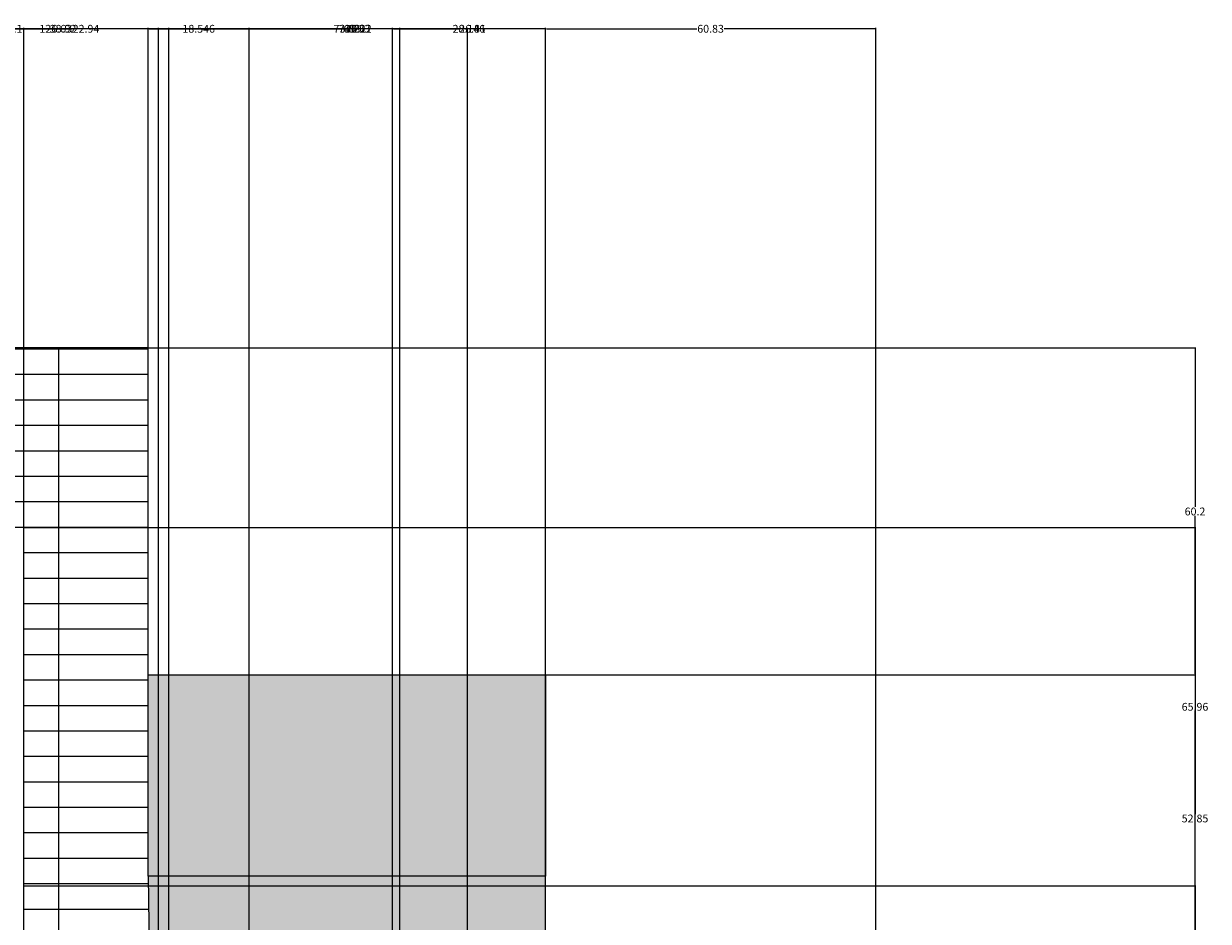
# Model space of a CAD drawing. Units: inches. Extents: x 241 to 943, y 109 to 1396.
# Tile 34 of 34: x 725 to 943, y 1231 to 1396. Entities that reach past the tile are written whole.
import ezdxf

# ---------------------------------------------------------------- set-up
doc = ezdxf.new("R2010")
doc.units = ezdxf.units.IN
doc.header["$MEASUREMENT"] = 0
for name, color, linetype, lineweight in [('A-ANNO-DIMS', 2, 'Continuous', 18), ('A-ELEV', 7, 'Continuous', 25), ('A-ELEV-SHAD', 9, 'Continuous', 13), ('A-WALL-PATT', 8, 'Continuous', 13)]:
    doc.layers.add(name, color=color, linetype=linetype, lineweight=lineweight)
doc.styles.get("Standard").update_dxf_attribs({"font": 'arial.ttf'})
doc.dimstyles.get("Standard").update_dxf_attribs({"dimtxt": 1.4375, "dimasz": 0.18, "dimexe": 0.18, "dimexo": 0.0625, "dimgap": 0.09, "dimtad": 0, "dimtih": 1, "dimtoh": 1, "dimdec": 4, "dimzin": 0, "dimdsep": 46, "dimlunit": 4, "dimtxsty": 'Standard', "dimcen": 0.09, "dimadec": 0, "dimazin": 0, "dimtfac": 1, "dimtdec": 4, "dimtofl": 0, "dimtmove": 0, "dimatfit": 3, "dimfxl": 1, "dimtolj": 1, "dimtzin": 0, "dimarcsym": 0})

# ---------------------------------------------------------------- blocks, each defined once
blk = doc.blocks.new('*D6')
at = {"layer": 'A-ANNO-DIMS', "color": 0, "lineweight": -2, "transparency": 16777216}
for p, q in [((820.84, 232.89), (820.84, 1395.05)), ((821.02, 1394.87), (848.73, 1394.87)), ((881.49, 1394.87), (853.77, 1394.87)), ((881.67, 232.89), (881.67, 1395.05))]:
    blk.add_line(p, q, dxfattribs=at)
at = {"layer": 'A-ANNO-DIMS', "color": 0, "transparency": 16777216}
for points in [[(821.02, 1394.9), (821.02, 1394.84), (820.84, 1394.87)], [(881.49, 1394.9), (881.49, 1394.84), (881.67, 1394.87)]]:
    blk.add_solid(points, dxfattribs=at)
at = {"layer": 'Defpoints', "color": 0, "transparency": 16777216}
for p in [(881.67, 1394.87), (820.84, 232.83), (881.67, 232.83)]:
    blk.add_point(p, dxfattribs=at)
at = {"layer": 'A-ANNO-DIMS', "color": 0, "transparency": 16777216, "insert": (851.25, 1394.87), "char_height": 1.438, "attachment_point": 5}
blk.add_mtext('\\A1;60.83', dxfattribs=at)
blk = doc.blocks.new('*D14')
at = {"layer": 'A-ANNO-DIMS', "color": 0, "lineweight": -2, "transparency": 16777216}
for p, q in [((667.39, 290.06), (667.39, 1395.05)), ((667.57, 1394.87), (727.7, 1394.87)), ((793.85, 1394.87), (733.72, 1394.87)), ((794.03, 290.06), (794.03, 1395.05))]:
    blk.add_line(p, q, dxfattribs=at)
at = {"layer": 'A-ANNO-DIMS', "color": 0, "transparency": 16777216}
for points in [[(667.57, 1394.9), (667.57, 1394.84), (667.39, 1394.87)], [(793.85, 1394.9), (793.85, 1394.84), (794.03, 1394.87)]]:
    blk.add_solid(points, dxfattribs=at)
at = {"layer": 'Defpoints', "color": 0, "transparency": 16777216}
for p in [(794.03, 1394.87), (667.39, 290), (794.03, 290)]:
    blk.add_point(p, dxfattribs=at)
at = {"layer": 'A-ANNO-DIMS', "color": 0, "transparency": 16777216, "insert": (730.71, 1394.87), "char_height": 1.438, "attachment_point": 5}
blk.add_mtext('\\A1;126.63', dxfattribs=at)
blk = doc.blocks.new('*D15')
at = {"layer": 'A-ANNO-DIMS', "color": 0, "lineweight": -2, "transparency": 16777216}
for p, q in [((794.03, 290.06), (794.03, 1395.05)), ((794.21, 1394.87), (805.04, 1394.87)), ((820.66, 1394.87), (809.82, 1394.87)), ((820.84, 232.89), (820.84, 1395.05))]:
    blk.add_line(p, q, dxfattribs=at)
at = {"layer": 'A-ANNO-DIMS', "color": 0, "transparency": 16777216}
for points in [[(794.21, 1394.9), (794.21, 1394.84), (794.03, 1394.87)], [(820.66, 1394.9), (820.66, 1394.84), (820.84, 1394.87)]]:
    blk.add_solid(points, dxfattribs=at)
at = {"layer": 'Defpoints', "color": 0, "transparency": 16777216}
for p in [(820.84, 1394.87), (794.03, 290), (820.84, 232.83)]:
    blk.add_point(p, dxfattribs=at)
at = {"layer": 'A-ANNO-DIMS', "color": 0, "transparency": 16777216, "insert": (807.43, 1394.87), "char_height": 1.438, "attachment_point": 5}
blk.add_mtext('\\A1;26.81', dxfattribs=at)
blk = doc.blocks.new('*D18')
at = {"layer": 'A-ANNO-DIMS', "color": 0, "lineweight": -2, "transparency": 16777216}
for p, q in [((508.31, 1336.18), (508.31, 1395.05)), ((508.49, 1394.87), (624.94, 1394.87)), ((747.58, 1394.87), (631.12, 1394.87)), ((747.76, 1336.18), (747.76, 1395.05))]:
    blk.add_line(p, q, dxfattribs=at)
at = {"layer": 'A-ANNO-DIMS', "color": 0, "transparency": 16777216}
for points in [[(508.49, 1394.9), (508.49, 1394.84), (508.31, 1394.87)], [(747.58, 1394.9), (747.58, 1394.84), (747.76, 1394.87)]]:
    blk.add_solid(points, dxfattribs=at)
at = {"layer": 'Defpoints', "color": 0, "transparency": 16777216}
for p in [(747.76, 1394.87), (508.31, 1336.12), (747.76, 1336.12)]:
    blk.add_point(p, dxfattribs=at)
at = {"layer": 'A-ANNO-DIMS', "color": 0, "transparency": 16777216, "insert": (628.03, 1394.87), "char_height": 1.438, "attachment_point": 5}
blk.add_mtext('\\A1;239.45', dxfattribs=at)
blk = doc.blocks.new('*D19')
at = {"layer": 'A-ANNO-DIMS', "color": 0, "lineweight": -2, "transparency": 16777216}
for p, q in [((747.76, 1275.98), (747.76, 1395.05)), ((747.94, 1394.87), (781.79, 1394.87)), ((820.66, 1394.87), (786.81, 1394.87)), ((820.84, 1275.98), (820.84, 1395.05))]:
    blk.add_line(p, q, dxfattribs=at)
at = {"layer": 'A-ANNO-DIMS', "color": 0, "transparency": 16777216}
for points in [[(747.94, 1394.9), (747.94, 1394.84), (747.76, 1394.87)], [(820.66, 1394.9), (820.66, 1394.84), (820.84, 1394.87)]]:
    blk.add_solid(points, dxfattribs=at)
at = {"layer": 'Defpoints', "color": 0, "transparency": 16777216}
for p in [(820.84, 1394.87), (747.76, 1275.91), (820.84, 1275.91)]:
    blk.add_point(p, dxfattribs=at)
at = {"layer": 'A-ANNO-DIMS', "color": 0, "transparency": 16777216, "insert": (784.3, 1394.87), "char_height": 1.438, "attachment_point": 5}
blk.add_mtext('\\A1;73.08', dxfattribs=at)
blk = doc.blocks.new('*D42')
at = {"layer": 'A-ANNO-DIMS', "color": 0, "lineweight": -2, "transparency": 16777216}
for p, q in [((820.9, 1275.91), (940.6, 1275.91)), ((940.42, 1275.73), (940.42, 1250.31)), ((940.42, 1223.24), (940.42, 1248.66)), ((820.9, 1223.06), (940.6, 1223.06))]:
    blk.add_line(p, q, dxfattribs=at)
at = {"layer": 'A-ANNO-DIMS', "color": 0, "transparency": 16777216}
for points in [[(940.39, 1275.73), (940.45, 1275.73), (940.42, 1275.91)], [(940.39, 1223.24), (940.45, 1223.24), (940.42, 1223.06)]]:
    blk.add_solid(points, dxfattribs=at)
at = {"layer": 'Defpoints', "color": 0, "transparency": 16777216}
for p in [(820.84, 1275.91), (940.42, 1275.91), (820.84, 1223.06)]:
    blk.add_point(p, dxfattribs=at)
at = {"layer": 'A-ANNO-DIMS', "color": 0, "transparency": 16777216, "insert": (940.42, 1249.49), "char_height": 1.438, "attachment_point": 5}
blk.add_mtext('\\A1;52.85', dxfattribs=at)
blk = doc.blocks.new('*D43')
at = {"layer": 'A-ANNO-DIMS', "color": 0, "lineweight": -2, "transparency": 16777216}
for p, q in [((747.82, 1336.12), (940.6, 1336.12)), ((940.42, 1335.94), (940.42, 1306.84)), ((940.42, 1276.09), (940.42, 1305.19)), ((747.82, 1275.91), (940.6, 1275.91))]:
    blk.add_line(p, q, dxfattribs=at)
at = {"layer": 'A-ANNO-DIMS', "color": 0, "transparency": 16777216}
for points in [[(940.39, 1335.94), (940.45, 1335.94), (940.42, 1336.12)], [(940.39, 1276.09), (940.45, 1276.09), (940.42, 1275.91)]]:
    blk.add_solid(points, dxfattribs=at)
at = {"layer": 'Defpoints', "color": 0, "transparency": 16777216}
for p in [(747.76, 1336.12), (940.42, 1336.12), (747.76, 1275.91)]:
    blk.add_point(p, dxfattribs=at)
at = {"layer": 'A-ANNO-DIMS', "color": 0, "transparency": 16777216, "insert": (940.42, 1306.01), "char_height": 1.438, "attachment_point": 5}
blk.add_mtext('\\A1;60.2', dxfattribs=at)
blk = doc.blocks.new('*D54')
at = {"layer": 'A-ANNO-DIMS', "color": 0, "lineweight": -2, "transparency": 16777216}
for p, q in [((724.88, 1237.07), (940.6, 1237.07)), ((940.42, 1236.89), (940.42, 1208.23)), ((940.42, 1177.91), (940.42, 1206.58)), ((724.88, 1177.73), (940.6, 1177.73))]:
    blk.add_line(p, q, dxfattribs=at)
at = {"layer": 'A-ANNO-DIMS', "color": 0, "transparency": 16777216}
for points in [[(940.39, 1236.89), (940.45, 1236.89), (940.42, 1237.07)], [(940.39, 1177.91), (940.45, 1177.91), (940.42, 1177.73)]]:
    blk.add_solid(points, dxfattribs=at)
at = {"layer": 'Defpoints', "color": 0, "transparency": 16777216}
for p in [(724.82, 1237.07), (940.42, 1237.07), (724.82, 1177.73)]:
    blk.add_point(p, dxfattribs=at)
at = {"layer": 'A-ANNO-DIMS', "color": 0, "transparency": 16777216, "insert": (940.42, 1207.4), "char_height": 1.438, "attachment_point": 5}
blk.add_mtext('\\A1;59.34', dxfattribs=at)
blk = doc.blocks.new('*D55')
at = {"layer": 'A-ANNO-DIMS', "color": 0, "lineweight": -2, "transparency": 16777216}
for p, q in [((724.88, 1303.03), (940.6, 1303.03)), ((940.42, 1302.85), (940.42, 1270.87)), ((940.42, 1237.25), (940.42, 1269.23)), ((724.88, 1237.07), (940.6, 1237.07))]:
    blk.add_line(p, q, dxfattribs=at)
at = {"layer": 'A-ANNO-DIMS', "color": 0, "transparency": 16777216}
for points in [[(940.39, 1302.85), (940.45, 1302.85), (940.42, 1303.03)], [(940.39, 1237.25), (940.45, 1237.25), (940.42, 1237.07)]]:
    blk.add_solid(points, dxfattribs=at)
at = {"layer": 'Defpoints', "color": 0, "transparency": 16777216}
for p in [(724.82, 1303.03), (940.42, 1303.03), (724.82, 1237.07)]:
    blk.add_point(p, dxfattribs=at)
at = {"layer": 'A-ANNO-DIMS', "color": 0, "transparency": 16777216, "insert": (940.42, 1270.05), "char_height": 1.438, "attachment_point": 5}
blk.add_mtext('\\A1;65.96', dxfattribs=at)
blk = doc.blocks.new('*D56')
at = {"layer": 'A-ANNO-DIMS', "color": 0, "lineweight": -2, "transparency": 16777216}
for p, q in [((533.95, 1303.09), (533.95, 1395.05)), ((534.13, 1394.87), (626.38, 1394.87)), ((724.64, 1394.87), (632.39, 1394.87)), ((724.82, 1303.09), (724.82, 1395.05))]:
    blk.add_line(p, q, dxfattribs=at)
at = {"layer": 'A-ANNO-DIMS', "color": 0, "transparency": 16777216}
for points in [[(534.13, 1394.9), (534.13, 1394.84), (533.95, 1394.87)], [(724.64, 1394.9), (724.64, 1394.84), (724.82, 1394.87)]]:
    blk.add_solid(points, dxfattribs=at)
at = {"layer": 'Defpoints', "color": 0, "transparency": 16777216}
for p in [(724.82, 1394.87), (533.95, 1303.03), (724.82, 1303.03)]:
    blk.add_point(p, dxfattribs=at)
at = {"layer": 'A-ANNO-DIMS', "color": 0, "transparency": 16777216, "insert": (629.39, 1394.87), "char_height": 1.438, "attachment_point": 5}
blk.add_mtext('\\A1;190.87', dxfattribs=at)
blk = doc.blocks.new('*D58')
at = {"layer": 'A-ANNO-DIMS', "color": 0, "lineweight": -2, "transparency": 16777216}
for p, q in [((766.3, 1177.6), (766.3, 1395.05)), ((766.48, 1394.87), (783.88, 1394.87)), ((806.35, 1394.87), (788.95, 1394.87)), ((806.53, 1177.6), (806.53, 1395.05))]:
    blk.add_line(p, q, dxfattribs=at)
at = {"layer": 'A-ANNO-DIMS', "color": 0, "transparency": 16777216}
for points in [[(766.48, 1394.9), (766.48, 1394.84), (766.3, 1394.87)], [(806.35, 1394.9), (806.35, 1394.84), (806.53, 1394.87)]]:
    blk.add_solid(points, dxfattribs=at)
at = {"layer": 'Defpoints', "color": 0, "transparency": 16777216}
for p in [(806.53, 1394.87), (766.3, 1177.54), (806.53, 1177.54)]:
    blk.add_point(p, dxfattribs=at)
at = {"layer": 'A-ANNO-DIMS', "color": 0, "transparency": 16777216, "insert": (786.42, 1394.87), "char_height": 1.438, "attachment_point": 5}
blk.add_mtext('\\A1;40.22', dxfattribs=at)
blk = doc.blocks.new('*D63')
at = {"layer": 'A-ANNO-DIMS', "color": 0, "lineweight": -2, "transparency": 16777216}
for p, q in [((651.6, 568.89), (651.6, 1395.05)), ((651.78, 1394.87), (719.84, 1394.87)), ((792.51, 1394.87), (724.45, 1394.87)), ((792.69, 568.89), (792.69, 1395.05))]:
    blk.add_line(p, q, dxfattribs=at)
at = {"layer": 'A-ANNO-DIMS', "color": 0, "transparency": 16777216}
for points in [[(651.78, 1394.9), (651.78, 1394.84), (651.6, 1394.87)], [(792.51, 1394.9), (792.51, 1394.84), (792.69, 1394.87)]]:
    blk.add_solid(points, dxfattribs=at)
at = {"layer": 'Defpoints', "color": 0, "transparency": 16777216}
for p in [(792.69, 1394.87), (651.6, 568.83), (792.69, 568.83)]:
    blk.add_point(p, dxfattribs=at)
at = {"layer": 'A-ANNO-DIMS', "color": 0, "transparency": 16777216, "insert": (722.14, 1394.87), "char_height": 1.438, "attachment_point": 5}
blk.add_mtext('\\A1;141.1', dxfattribs=at)
blk = doc.blocks.new('*D64')
at = {"layer": 'A-ANNO-DIMS', "color": 0, "lineweight": -2, "transparency": 16777216}
for p, q in [((792.69, 568.89), (792.69, 1395.05)), ((792.87, 1394.87), (803.68, 1394.87)), ((820.66, 1394.87), (809.85, 1394.87)), ((820.84, 568.89), (820.84, 1395.05))]:
    blk.add_line(p, q, dxfattribs=at)
at = {"layer": 'A-ANNO-DIMS', "color": 0, "transparency": 16777216}
for points in [[(792.87, 1394.9), (792.87, 1394.84), (792.69, 1394.87)], [(820.66, 1394.9), (820.66, 1394.84), (820.84, 1394.87)]]:
    blk.add_solid(points, dxfattribs=at)
at = {"layer": 'Defpoints', "color": 0, "transparency": 16777216}
for p in [(820.84, 1394.87), (792.69, 568.83), (820.84, 568.83)]:
    blk.add_point(p, dxfattribs=at)
at = {"layer": 'A-ANNO-DIMS', "color": 0, "transparency": 16777216, "insert": (806.76, 1394.87), "char_height": 1.438, "attachment_point": 5}
blk.add_mtext('\\A1;28.146', dxfattribs=at)
blk = doc.blocks.new('*D66')
at = {"layer": 'A-ANNO-DIMS', "color": 0, "lineweight": -2, "transparency": 16777216}
for p, q in [((617.76, 702.85), (617.76, 1395.05)), ((617.94, 1394.87), (680.69, 1394.87)), ((749.45, 1394.87), (686.7, 1394.87)), ((749.63, 702.85), (749.63, 1395.05))]:
    blk.add_line(p, q, dxfattribs=at)
at = {"layer": 'A-ANNO-DIMS', "color": 0, "transparency": 16777216}
for points in [[(617.94, 1394.9), (617.94, 1394.84), (617.76, 1394.87)], [(749.45, 1394.9), (749.45, 1394.84), (749.63, 1394.87)]]:
    blk.add_solid(points, dxfattribs=at)
at = {"layer": 'Defpoints', "color": 0, "transparency": 16777216}
for p in [(749.63, 1394.87), (617.76, 702.79), (749.63, 702.79)]:
    blk.add_point(p, dxfattribs=at)
at = {"layer": 'A-ANNO-DIMS', "color": 0, "transparency": 16777216, "insert": (683.7, 1394.87), "char_height": 1.438, "attachment_point": 5}
blk.add_mtext('\\A1;131.87', dxfattribs=at)
blk = doc.blocks.new('*D68')
at = {"layer": 'A-ANNO-DIMS', "color": 0, "lineweight": -2, "transparency": 16777216}
for p, q in [((617.76, 841.6), (617.76, 1395.05)), ((617.94, 1394.87), (702.22, 1394.87)), ((792.51, 1394.87), (708.23, 1394.87)), ((792.69, 841.6), (792.69, 1395.05))]:
    blk.add_line(p, q, dxfattribs=at)
at = {"layer": 'A-ANNO-DIMS', "color": 0, "transparency": 16777216}
for points in [[(617.94, 1394.9), (617.94, 1394.84), (617.76, 1394.87)], [(792.51, 1394.9), (792.51, 1394.84), (792.69, 1394.87)]]:
    blk.add_solid(points, dxfattribs=at)
at = {"layer": 'Defpoints', "color": 0, "transparency": 16777216}
for p in [(792.69, 1394.87), (617.76, 841.54), (792.69, 841.54)]:
    blk.add_point(p, dxfattribs=at)
at = {"layer": 'A-ANNO-DIMS', "color": 0, "transparency": 16777216, "insert": (705.23, 1394.87), "char_height": 1.438, "attachment_point": 5}
blk.add_mtext('\\A1;174.93', dxfattribs=at)
blk = doc.blocks.new('*D70')
at = {"layer": 'A-ANNO-DIMS', "color": 0, "lineweight": -2, "transparency": 16777216}
for p, q in [((603.87, 1009.6), (603.87, 1395.05)), ((604.05, 1394.87), (674.69, 1394.87)), ((751.33, 1394.87), (680.69, 1394.87)), ((751.51, 1009.6), (751.51, 1395.05))]:
    blk.add_line(p, q, dxfattribs=at)
at = {"layer": 'A-ANNO-DIMS', "color": 0, "transparency": 16777216}
for points in [[(604.05, 1394.9), (604.05, 1394.84), (603.87, 1394.87)], [(751.33, 1394.9), (751.33, 1394.84), (751.51, 1394.87)]]:
    blk.add_solid(points, dxfattribs=at)
at = {"layer": 'Defpoints', "color": 0, "transparency": 16777216}
for p in [(751.51, 1394.87), (603.87, 1009.54), (751.51, 1009.54)]:
    blk.add_point(p, dxfattribs=at)
at = {"layer": 'A-ANNO-DIMS', "color": 0, "transparency": 16777216, "insert": (677.69, 1394.87), "char_height": 1.438, "attachment_point": 5}
blk.add_mtext('\\A1;147.64', dxfattribs=at)
blk = doc.blocks.new('*D71')
at = {"layer": 'A-ANNO-DIMS', "color": 0, "lineweight": -2, "transparency": 16777216}
for p, q in [((751.51, 902.92), (751.51, 1395.05)), ((751.69, 1394.87), (783.65, 1394.87)), ((820.66, 1394.87), (788.69, 1394.87)), ((820.84, 902.92), (820.84, 1395.05))]:
    blk.add_line(p, q, dxfattribs=at)
at = {"layer": 'A-ANNO-DIMS', "color": 0, "transparency": 16777216}
for points in [[(751.69, 1394.9), (751.69, 1394.84), (751.51, 1394.87)], [(820.66, 1394.9), (820.66, 1394.84), (820.84, 1394.87)]]:
    blk.add_solid(points, dxfattribs=at)
at = {"layer": 'Defpoints', "color": 0, "transparency": 16777216}
for p in [(820.84, 1394.87), (751.51, 902.85), (820.84, 902.85)]:
    blk.add_point(p, dxfattribs=at)
at = {"layer": 'A-ANNO-DIMS', "color": 0, "transparency": 16777216, "insert": (786.17, 1394.87), "char_height": 1.438, "attachment_point": 5}
blk.add_mtext('\\A1;69.33', dxfattribs=at)
blk = doc.blocks.new('*D84')
at = {"layer": 'A-ANNO-DIMS', "color": 0, "lineweight": -2, "transparency": 16777216}
for p, q in [((749.63, 702.85), (749.63, 1395.05)), ((749.81, 1394.87), (782.73, 1394.87)), ((820.66, 1394.87), (787.74, 1394.87)), ((820.84, 736.89), (820.84, 1395.05))]:
    blk.add_line(p, q, dxfattribs=at)
at = {"layer": 'A-ANNO-DIMS', "color": 0, "transparency": 16777216}
for points in [[(749.81, 1394.9), (749.81, 1394.84), (749.63, 1394.87)], [(820.66, 1394.9), (820.66, 1394.84), (820.84, 1394.87)]]:
    blk.add_solid(points, dxfattribs=at)
at = {"layer": 'Defpoints', "color": 0, "transparency": 16777216}
for p in [(820.84, 1394.87), (820.84, 736.83), (749.63, 702.79)]:
    blk.add_point(p, dxfattribs=at)
at = {"layer": 'A-ANNO-DIMS', "color": 0, "transparency": 16777216, "insert": (785.24, 1394.87), "char_height": 1.438, "attachment_point": 5}
blk.add_mtext('\\A1;71.20', dxfattribs=at)
blk = doc.blocks.new('*D93')
at = {"layer": 'A-ANNO-DIMS', "color": 0, "lineweight": -2, "transparency": 16777216}
for p, q in [((724.82, 1303.09), (724.82, 1395.05)), ((725, 1394.87), (733.76, 1394.87)), ((747.58, 1394.87), (738.81, 1394.87)), ((747.76, 1275.98), (747.76, 1395.05))]:
    blk.add_line(p, q, dxfattribs=at)
at = {"layer": 'A-ANNO-DIMS', "color": 0, "transparency": 16777216}
for points in [[(725, 1394.9), (725, 1394.84), (724.82, 1394.87)], [(747.58, 1394.9), (747.58, 1394.84), (747.76, 1394.87)]]:
    blk.add_solid(points, dxfattribs=at)
at = {"layer": 'Defpoints', "color": 0, "transparency": 16777216}
for p in [(747.76, 1394.87), (724.82, 1303.03), (747.76, 1275.91)]:
    blk.add_point(p, dxfattribs=at)
at = {"layer": 'A-ANNO-DIMS', "color": 0, "transparency": 16777216, "insert": (736.29, 1394.87), "char_height": 1.438, "attachment_point": 5}
blk.add_mtext('\\A1;22.94', dxfattribs=at)
blk = doc.blocks.new('*D94')
at = {"layer": 'A-ANNO-DIMS', "color": 0, "lineweight": -2, "transparency": 16777216}
for p, q in [((747.76, 1275.98), (747.76, 1395.05)), ((747.94, 1394.87), (754.03, 1394.87)), ((766.12, 1394.87), (760.04, 1394.87)), ((766.3, 1103.11), (766.3, 1395.05))]:
    blk.add_line(p, q, dxfattribs=at)
at = {"layer": 'A-ANNO-DIMS', "color": 0, "transparency": 16777216}
for points in [[(747.94, 1394.9), (747.94, 1394.84), (747.76, 1394.87)], [(766.12, 1394.9), (766.12, 1394.84), (766.3, 1394.87)]]:
    blk.add_solid(points, dxfattribs=at)
at = {"layer": 'Defpoints', "color": 0, "transparency": 16777216}
for p in [(766.3, 1394.87), (747.76, 1275.91), (766.3, 1103.05)]:
    blk.add_point(p, dxfattribs=at)
at = {"layer": 'A-ANNO-DIMS', "color": 0, "transparency": 16777216, "insert": (757.03, 1394.87), "char_height": 1.438, "attachment_point": 5}
blk.add_mtext('\\A1;18.546', dxfattribs=at)
blk = doc.blocks.new('*D109')
at = {"layer": 'A-ANNO-DIMS', "color": 0, "lineweight": -2, "transparency": 16777216}
for p, q in [((682.87, 1110.23), (682.87, 1395.05)), ((683.05, 1394.87), (701.31, 1394.87)), ((724.64, 1394.87), (706.39, 1394.87)), ((724.82, 1108.23), (724.82, 1395.05))]:
    blk.add_line(p, q, dxfattribs=at)
at = {"layer": 'A-ANNO-DIMS', "color": 0, "transparency": 16777216}
for points in [[(683.05, 1394.9), (683.05, 1394.84), (682.87, 1394.87)], [(724.64, 1394.9), (724.64, 1394.84), (724.82, 1394.87)]]:
    blk.add_solid(points, dxfattribs=at)
at = {"layer": 'Defpoints', "color": 0, "transparency": 16777216}
for p in [(724.82, 1394.87), (682.87, 1110.17), (724.82, 1108.17)]:
    blk.add_point(p, dxfattribs=at)
at = {"layer": 'A-ANNO-DIMS', "color": 0, "transparency": 16777216, "insert": (703.85, 1394.87), "char_height": 1.438, "attachment_point": 5}
blk.add_mtext('\\A1;41.94', dxfattribs=at)
blk = doc.blocks.new('*D117')
at = {"layer": 'A-ANNO-DIMS', "color": 0, "lineweight": -2, "transparency": 16777216}
for p, q in [((712.58, 902.92), (712.58, 1395.05)), ((712.76, 1394.87), (729.54, 1394.87)), ((751.33, 1394.87), (734.55, 1394.87)), ((751.51, 902.92), (751.51, 1395.05))]:
    blk.add_line(p, q, dxfattribs=at)
at = {"layer": 'A-ANNO-DIMS', "color": 0, "transparency": 16777216}
for points in [[(712.76, 1394.9), (712.76, 1394.84), (712.58, 1394.87)], [(751.33, 1394.9), (751.33, 1394.84), (751.51, 1394.87)]]:
    blk.add_solid(points, dxfattribs=at)
at = {"layer": 'Defpoints', "color": 0, "transparency": 16777216}
for p in [(751.51, 1394.87), (712.58, 902.85), (751.51, 902.85)]:
    blk.add_point(p, dxfattribs=at)
at = {"layer": 'A-ANNO-DIMS', "color": 0, "transparency": 16777216, "insert": (732.05, 1394.87), "char_height": 1.438, "attachment_point": 5}
blk.add_mtext('\\A1;38.92', dxfattribs=at)

msp = doc.modelspace()

# ---------------------------------------------------------------- hatches: boundary and pattern name
at = {"layer": 'A-ELEV-SHAD'}
h = msp.add_hatch(color=256, dxfattribs=at)
h.dxf.hatch_style = 1
h.paths.add_polyline_path([(508.3064, 1070.8538), (377.0391, 1070.8538), (377.0391, 1009.5382), (508.3064, 1009.5382)])
h.paths.add_polyline_path([(508.3064, 1238.8538), (377.0391, 1238.8538), (377.0391, 1177.5382), (508.3064, 1177.5382)])
h.paths.add_polyline_path([(581.3632, 902.8538), (568.1348, 902.8538), (553.5166, 902.8538), (377.0391, 902.8538), (377.0391, 841.5382), (553.5166, 841.5382), (564.8076, 841.5382), (581.3632, 841.5382)])
h.paths.add_polyline_path([(820.8374, 1275.9142), (747.7579, 1275.9142), (747.7579, 1238.8538), (820.8374, 1238.8538)])
h.paths.add_polyline_path([(820.8374, 1238.8538), (747.7579, 1238.8538), (747.9341, 1223.0633), (820.8374, 1223.0633)])
h.paths.add_polyline_path([(396.3125, 841.5382), (377.0391, 841.5382), (377.0391, 734.8538), (389.0429, 734.8538), (389.0429, 735.188), (389.0429, 773.4916), (396.3125, 773.4916), (396.3125, 780.5808), (390.5597, 780.5808), (388.0428, 780.5808, -1), (388.0428, 782.5808), (390.5597, 782.5808), (396.3125, 782.5808)])
at = {"layer": 'A-WALL-PATT'}
h = msp.add_hatch(dxfattribs=at)
h.set_pattern_fill('GRATE', color=256, scale=150)
h.paths.add_polyline_path([(747.7579, 1238.8538), (747.7579, 1275.9142), (747.7579, 1336.1154), (508.3064, 1336.1154), (508.3064, 1275.9142), (508.3064, 1238.8538), (508.3064, 1177.5382), (508.3064, 1109.4916), (508.3064, 1070.8538), (553.5166, 1070.8538), (749.6328, 1070.8538)])
h.paths.add_polyline_path([(533.952, 1108.1686), (533.952, 1177.7336), (533.952, 1303.0286), (724.819, 1303.0286), (724.819, 1108.1686)], flags=16)
h.paths.add_polyline_path([(535.952, 1110.1686), (535.952, 1175.7336), (722.819, 1175.7336), (722.819, 1110.1686)], flags=0)
h.paths.add_polyline_path([(643.4534, 1134.0739), (622.521, 1134.0739), (622.521, 1136.0739), (643.4534, 1136.0739)], flags=0)
h.paths.add_polyline_path([(617.7594, 568.8295), (617.7594, 734.8538), (377.0391, 734.8538), (377.0391, 566.8538), (377.0391, 400.8295), (417.0913, 400.8295), (618.9643, 400.8295)])
h.paths.add_polyline_path([(424.1086, 496.4395), (424.1086, 568.8295), (565.2023, 568.8295), (565.2023, 496.4395)], flags=16)
h.paths.add_polyline_path([(426.1086, 498.4395), (426.1086, 566.8295), (563.2023, 566.8295), (563.2023, 508.9074), (563.2023, 498.4395)], flags=0)
h.paths.add_polyline_path([(508.0803, 508.9074), (508.0803, 519.3754), (450.9259, 519.3754), (450.9259, 525.3816), (445.5808, 525.3816, -1), (445.5808, 527.3816), (450.9259, 527.3816), (450.9259, 566.8295), (508.0803, 566.8295), (537.4269, 566.8295), (537.4269, 508.9074)], flags=0)
h.paths.add_polyline_path([(506.0803, 521.3754), (452.9259, 521.3754), (452.9259, 564.8295), (506.0803, 564.8295)], flags=0)
h.paths.add_polyline_path([(424.1086, 628.4013), (424.1086, 700.7912), (592.9542, 700.7912), (592.9542, 628.4013)], flags=16)
h.paths.add_polyline_path([(426.1086, 630.4013), (426.1086, 698.7912), (590.8792, 698.7912), (590.8792, 630.4013)], flags=0)
h.paths.add_polyline_path([(508.1906, 651.3371), (508.0803, 651.3371), (450.9259, 651.3371), (428.0291, 651.3371), (428.0291, 698.7912), (451.9767, 698.7912), (508.0803, 698.7912), (537.4269, 698.7912), (563.2023, 698.7912), (563.2023, 659.3434), (563.9297, 659.3434), (563.9297, 651.3371)], flags=0)
h.paths.add_polyline_path([(506.0803, 653.3371), (452.9259, 653.3371), (452.9259, 657.3434), (445.5808, 657.3434, -1), (445.5808, 659.3434), (452.9259, 659.3434), (452.9259, 696.7912), (506.0803, 696.7912)], flags=0)

# ---------------------------------------------------------------- linework, layer by layer
at = {"layer": 'A-ELEV'}
for p, q in [((747.7579, 1336.1154), (508.3064, 1336.1154)), ((747.7579, 1275.9142), (747.7579, 1336.1154)), ((747.7579, 1238.8538), (747.7579, 1275.9142)), ((747.7579, 1275.9142), (820.8374, 1275.9142)), ((820.8374, 1275.9142), (820.8374, 1238.8538)), ((820.8374, 1238.8538), (747.7579, 1238.8538)), ((747.7579, 1238.8538), (749.6328, 1070.8538)), ((820.8374, 1070.8538), (820.8374, 1238.8538))]:
    msp.add_line(p, q, dxfattribs=at)

# ---------------------------------------------------------------- dimensions: what is measured, and where the dimension line sits
at = {"layer": 'A-ANNO-DIMS'}
for base, p1, p2, override, picture, middle in [((747.7579, 1394.8654), (508.3064, 1336.1154), (747.7579, 1336.1154), {"dimdec": 2, "dimlfac": 1, "dimrnd": 0, "dimzin": 0, "dimdsep": 46, "dimlunit": 2}, '*D18', (628.0322, 1394.8654)), ((724.819, 1394.8654), (533.952, 1303.0286), (724.819, 1303.0286), {"dimdec": 2, "dimlfac": 1, "dimrnd": 0, "dimzin": 0, "dimdsep": 46, "dimlunit": 2}, '*D56', (629.3855, 1394.8654)), ((751.5078, 1394.8654), (603.8694, 1009.5382), (751.5078, 1009.5382), {"dimdec": 2, "dimlfac": 1, "dimrnd": 0, "dimzin": 0, "dimdsep": 46, "dimlunit": 2}, '*D70', (677.6886, 1394.8654)), ((749.6328, 1394.8654), (617.7594, 702.7912), (749.6328, 702.7912), {"dimdec": 2, "dimlfac": 1, "dimrnd": 0, "dimzin": 0, "dimdsep": 46, "dimlunit": 2}, '*D66', (683.6961, 1394.8654)), ((792.691, 1394.8654), (617.7594, 841.5382), (792.691, 841.5382), {"dimdec": 2, "dimlfac": 1, "dimrnd": 0, "dimzin": 0, "dimdsep": 46, "dimlunit": 2}, '*D68', (705.2252, 1394.8654)), ((792.691, 1394.8654), (651.5974, 568.8295), (792.691, 568.8295), {"dimdec": 1, "dimlfac": 1, "dimrnd": 0, "dimzin": 0, "dimdsep": 46, "dimlunit": 2}, '*D63', (722.1442, 1394.8654)), ((794.0275, 1394.8654), (667.3935, 289.9984), (794.0275, 289.9984), {"dimdec": 2, "dimlfac": 1, "dimrnd": 0, "dimzin": 0, "dimdsep": 46, "dimlunit": 2}, '*D14', (730.7105, 1394.8654)), ((724.819, 1394.8654), (682.8748, 1110.1686), (724.819, 1108.1686), {"dimdec": 2, "dimlfac": 1, "dimrnd": 0, "dimzin": 0, "dimdsep": 46, "dimlunit": 2}, '*D109', (703.8469, 1394.8654)), ((751.5078, 1394.8654), (712.5839, 902.8538), (751.5078, 902.8538), {"dimdec": 2, "dimlfac": 1, "dimrnd": 0, "dimzin": 0, "dimdsep": 46, "dimlunit": 2}, '*D117', (732.0459, 1394.8654)), ((747.7579, 1394.8654), (724.819, 1303.0286), (747.7579, 1275.9142), {"dimdec": 2, "dimlfac": 1, "dimrnd": 0, "dimzin": 0, "dimdsep": 46, "dimlunit": 2}, '*D93', (736.2885, 1394.8654)), ((820.8374, 1394.8654), (747.7579, 1275.9142), (820.8374, 1275.9142), {"dimdec": 2, "dimlfac": 1, "dimrnd": 0, "dimzin": 0, "dimdsep": 46, "dimlunit": 2}, '*D19', (784.2976, 1394.8654)), ((766.3038, 1394.8654), (747.7579, 1275.9142), (766.3038, 1103.0477), {"dimdec": 3, "dimlfac": 1, "dimrnd": 0, "dimzin": 0, "dimdsep": 46, "dimlunit": 2}, '*D94', (757.0309, 1394.8654)), ((820.8374, 1394.8654), (749.6328, 702.7912), (820.8374, 736.8295), {"dimdec": 2, "dimlfac": 1, "dimrnd": 0, "dimzin": 0, "dimdsep": 46, "dimlunit": 2}, '*D84', (785.2351, 1394.8654)), ((820.8374, 1394.8654), (751.5078, 902.8538), (820.8374, 902.8538), {"dimdec": 2, "dimlfac": 1, "dimrnd": 0, "dimzin": 0, "dimdsep": 46, "dimlunit": 2}, '*D71', (786.1726, 1394.8654)), ((806.5268, 1394.8654), (766.3038, 1177.5382), (806.5268, 1177.5382), {"dimdec": 2, "dimlfac": 1, "dimrnd": 0, "dimzin": 0, "dimdsep": 46, "dimlunit": 2}, '*D58', (786.4153, 1394.8654)), ((820.8374, 1394.8654), (792.691, 568.8295), (820.8374, 568.8295), {"dimdec": 3, "dimlfac": 1, "dimrnd": 0, "dimzin": 0, "dimdsep": 46, "dimlunit": 2}, '*D64', (806.7642, 1394.8654)), ((820.8374, 1394.8654), (794.0275, 289.9984), (820.8374, 232.8295), {"dimdec": 2, "dimlfac": 1, "dimrnd": 0, "dimzin": 0, "dimdsep": 46, "dimlunit": 2}, '*D15', (807.4324, 1394.8654)), ((881.667, 1394.8654), (820.8374, 232.8295), (881.667, 232.8295), {"dimdec": 2, "dimlfac": 1, "dimrnd": 0, "dimzin": 0, "dimdsep": 46, "dimlunit": 2}, '*D6', (851.2522, 1394.8654))]:
    dim = msp.add_linear_dim(base=base, p1=p1, p2=p2, dimstyle='Standard', override=override, dxfattribs=at)
    dim.commit()
    dim.dimension.update_dxf_attribs({"geometry": picture, "text_midpoint": middle})
for base, p1, p2, override, picture, middle in [((940.417, 1336.1154), (747.7579, 1275.9142), (747.7579, 1336.1154), {"dimdec": 1, "dimlfac": 1, "dimrnd": 0, "dimzin": 0, "dimdsep": 46, "dimlunit": 2}, '*D43', (940.417, 1306.0148)), ((940.417, 1303.0286), (724.819, 1237.0695), (724.819, 1303.0286), {"dimdec": 2, "dimlfac": 1, "dimrnd": 0, "dimzin": 0, "dimdsep": 46, "dimlunit": 2}, '*D55', (940.417, 1270.049)), ((940.417, 1275.9142), (820.8374, 1223.0633), (820.8374, 1275.9142), {"dimdec": 2, "dimlfac": 1, "dimrnd": 0, "dimzin": 0, "dimdsep": 46, "dimlunit": 2}, '*D42', (940.417, 1249.4888)), ((940.417, 1237.0695), (724.819, 1177.7336), (724.819, 1237.0695), {"dimdec": 2, "dimlfac": 1, "dimrnd": 0, "dimzin": 0, "dimdsep": 46, "dimlunit": 2}, '*D54', (940.417, 1207.4016))]:
    dim = msp.add_linear_dim(base=base, p1=p1, p2=p2, angle=90, dimstyle='Standard', override=override, dxfattribs=at)
    dim.commit()
    dim.dimension.update_dxf_attribs({"geometry": picture, "text_midpoint": middle})

doc.saveas('drawing.dxf')
